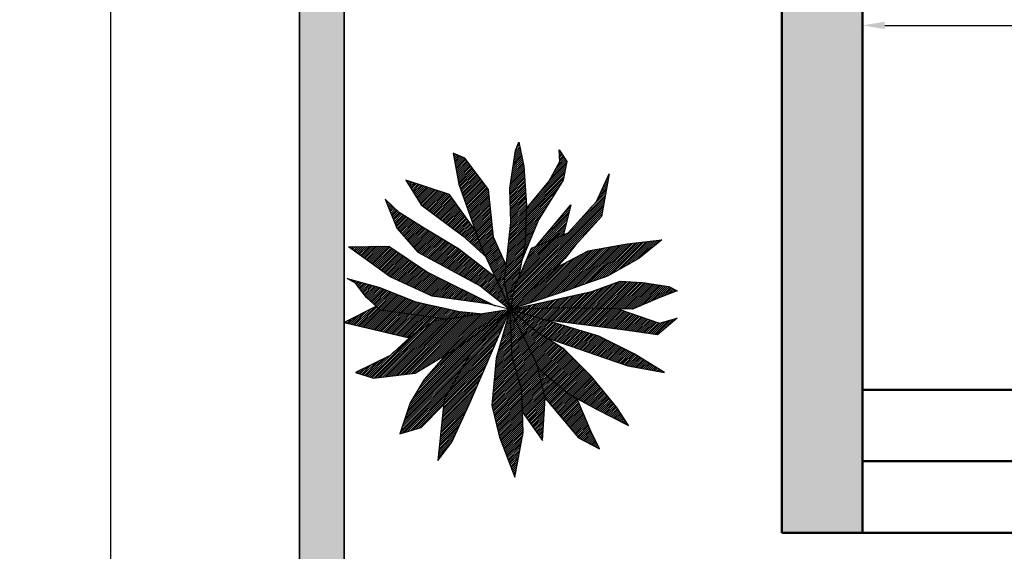
# Model space of a CAD drawing. Units: inches. Extents: x 3008 to 4088, y 1255 to 2137.
# Tile 3 of 30: x 3008 to 3119, y 1539 to 1598. Entities that reach past the tile are written whole.
import ezdxf

# ---------------------------------------------------------------- set-up
doc = ezdxf.new("R2010")
doc.units = ezdxf.units.IN
for name, color, linetype, lineweight in [('A-ANNO-DIMS', 2, 'Continuous', 18), ('A-WALL', 7, 'Continuous', 50), ('A-WALL-PATT', 8, 'Continuous', 13), ('C-PROP', 1, 'Continuous', 35), ('C-PROP-PATT', 9, 'Continuous', 13), ('L-PLNT', 3, 'Continuous', 13), ('vfolhas', 114, 'Continuous', 5)]:
    doc.layers.add(name, color=color, linetype=linetype, lineweight=lineweight)
for name, color, linetype in [('vfolha', 72, 'Continuous'), ('vfolha2', 110, 'Continuous'), ('vfolhas2', 102, 'Continuous')]:
    doc.layers.add(name, color=color, linetype=linetype)
doc.styles.get("Standard").update_dxf_attribs({"font": 'arial.ttf'})
doc.dimstyles.new('ISO-25', dxfattribs={"dimtxt": 8, "dimasz": 2.5, "dimexe": 1.25, "dimexo": 0.625, "dimtad": 1, "dimdec": 1, "dimlunit": 3, "dimtxsty": 'Standard', "dimcen": 2.5, "dimadec": 0, "dimazin": 0, "dimtfac": 1, "dimtdec": 1, "dimtmove": 0, "dimatfit": 3, "dimfxl": 1, "dimarcsym": 0})
pattern_1 = [(45, (-2446.5133113, 50.986076), (-0.004419417382, 0.004419417382), [])]

# ---------------------------------------------------------------- blocks, each defined once
blk = doc.blocks.new('*D2')
at = {"layer": 'A-ANNO-DIMS', "color": 0, "lineweight": -2, "transparency": 16777216}
for p, q in [((3039.04, 2003.97), (3017.26, 2003.97)), ((3018.51, 2001.47), (3018.51, 1346.47)), ((3039.04, 1343.97), (3017.26, 1343.97))]:
    blk.add_line(p, q, dxfattribs=at)
at = {"layer": 'A-ANNO-DIMS', "color": 0, "transparency": 16777216}
for points in [[(3018.09, 2001.47), (3018.93, 2001.47), (3018.51, 2003.97)], [(3018.09, 1346.47), (3018.93, 1346.47), (3018.51, 1343.97)]]:
    blk.add_solid(points, dxfattribs=at)
at = {"layer": 'Defpoints', "color": 0, "transparency": 16777216}
for p in [(3039.67, 2003.97), (3018.51, 1343.97), (3039.67, 1343.97)]:
    blk.add_point(p, dxfattribs=at)
at = {"layer": 'A-ANNO-DIMS', "color": 0, "transparency": 16777216, "insert": (3013.82, 1673.97), "char_height": 8, "attachment_point": 5, "rotation": 90}
blk.add_mtext("55'", dxfattribs=at)
blk = doc.blocks.new('arbusto_PB_verde_grande')
at = {"layer": 'vfolha2'}
h = blk.add_hatch(dxfattribs=at)
h.set_pattern_fill('ANSI31', color=256, scale=0.05, style=0)
h.set_pattern_definition(pattern_1)
h.paths.add_polyline_path([(0.0294, 0.3565), (0.0003, 0.0905), (0.0263, -0.0393), (0.047, 0.0623), (0.0619, 0.0973), (0.0937, 0.2657), (0.0996, 0.4347), (0.0879, 0.6131), (0.0645, 0.7227), (0.0499, 0.6851), (0.0236, 0.5129)])
h.paths.add_polyline_path([(0.3011, 0.4379), (0.1423, 0.2487), (0.2669, 0.3002)])
h.paths.add_polyline_path([(0.38, 0.2282), (0.237, 0.1519), (0.1843, 0.0936), (0.1112, 0.0436), (0.0263, -0.0393), (0.2806, 0.0467), (0.3683, 0.078), (0.4676, 0.1124), (0.6107, 0.1938), (0.7159, 0.2782), (0.5581, 0.2595)])
h.paths.add_polyline_path([(0.561, -0.2944), (0.7275, -0.3257), (0.5902, -0.2412), (0.4296, -0.1598), (0.0263, -0.0393), (0.1492, -0.1411), (0.1884, -0.166), (0.415, -0.2444)])
h.paths.add_polyline_path([(-0.2743, -0.4478), (-0.3035, -0.7263), (-0.2392, -0.6417), (-0.1546, -0.4572), (0.0263, -0.0393), (-0.1633, -0.2538)])
h.paths.add_polyline_path([(-0.5196, -0.2474), (-0.6774, -0.3257), (-0.5956, -0.3507), (-0.4057, -0.3288), (-0.2101, -0.21), (0.0263, -0.0393), (-0.1487, -0.0659), (-0.3152, -0.091), (-0.4145, -0.1505)])
h.paths.add_polyline_path([(-0.5255, 0.2501), (-0.7095, 0.247), (-0.5196, 0.1093), (-0.3298, 0.0217), (-0.0757, -0.0128), (-0.0423, -0.0215), (-0.3502, 0.1312)])
h = blk.add_hatch(dxfattribs=at)
h.set_pattern_fill('ANSI31', color=256, scale=0.05, style=0)
h.set_pattern_definition(pattern_1)
h.paths.add_polyline_path([(-0.1896, 0.297), (-0.0855, 0.2019), (-0.1078, 0.2501), (-0.132, 0.3187), (-0.251, 0.4848), (-0.4495, 0.5505), (-0.3795, 0.4379)])
h.paths.add_polyline_path([(0.0791, -0.4071), (0.0821, -0.5063), (0.1726, -0.6355), (0.1843, -0.4415), (0.149, -0.2918), (0.0263, -0.0393), (0.0353, -0.2538)])
at = {"layer": 'vfolhas'}
h = blk.add_hatch(dxfattribs=at)
h.set_pattern_fill('ANSI31', color=256, scale=0.05, style=0)
h.set_pattern_definition(pattern_1)
h.paths.add_polyline_path([(-0.0728, 0.5067), (-0.1808, 0.6506), (-0.2334, 0.6725), (-0.2071, 0.5318), (-0.1078, 0.2501), (0.0263, -0.0393), (0.0003, 0.0905), (0.0082, 0.1624), (-0.0494, 0.2908)])
h.paths.add_polyline_path([(0.099, 0.4193), (0.0937, 0.2657), (0.0791, 0.1881), (0.1551, 0.369), (0.2661, 0.5505), (0.2836, 0.635), (0.2485, 0.6882), (0.2514, 0.635), (0.2018, 0.5443)])
h.paths.add_polyline_path([(0.1229, 0.2407), (0.047, 0.0623), (0.0263, -0.0393), (0.1112, 0.0436), (0.1843, 0.0936), (0.2748, 0.1938), (0.3215, 0.2532), (0.4413, 0.3847), (0.4763, 0.5787), (0.4179, 0.4535), (0.2894, 0.3095)])
h.paths.add_polyline_path([(0.5815, -0.0378), (0.7071, 0.0154), (0.7859, 0.0467), (0.748, 0.0655), (0.6282, 0.0842), (0.526, 0.0905), (0.3974, 0.0436), (0.0263, -0.0393), (0.2573, -0.0315), (0.4383, -0.0347)])
h.paths.add_polyline_path([(0.5202, -0.0365), (0.4383, -0.0347), (0.2573, -0.0315), (0.0263, -0.0393), (0.1796, -0.0852), (0.5377, -0.1317), (0.6954, -0.1536), (0.7859, -0.0785), (0.7041, -0.1004)])
h.paths.add_polyline_path([(0.2719, -0.2193), (0.1492, -0.1411), (0.0263, -0.0393), (0.1579, -0.3101), (0.2952, -0.4258), (0.4179, -0.4916), (0.564, -0.5667), (0.5114, -0.4853), (0.3946, -0.3414)])
h.paths.add_polyline_path([(-0.0582, -0.4759), (-0.0231, -0.6198), (0.047, -0.8013), (0.0849, -0.5979), (0.0791, -0.4071), (0.0353, -0.2538), (0.0263, -0.0393), (-0.0377, -0.26)])
h.paths.add_polyline_path([(-0.2422, 0.1405), (-0.1107, 0.0686), (0.0263, -0.0393), (-0.0423, 0.1087), (-0.2101, 0.2376), (-0.3649, 0.3314), (-0.4787, 0.4034), (-0.543, 0.4629), (-0.4904, 0.3314), (-0.3941, 0.2219)])
h = blk.add_hatch(dxfattribs=at)
h.set_pattern_fill('ANSI31', color=256, scale=0.05, style=0)
h.set_pattern_definition(pattern_1)
h.paths.add_polyline_path([(-0.5722, 0.0623), (-0.7153, 0.103), (-0.6774, 0.0811), (-0.6277, 0.0154), (-0.5635, -0.041), (-0.2646, -0.0834), (-0.1487, -0.0659), (-0.1015, -0.0588), (-0.2042, -0.0472), (-0.4028, -0.0034)])
h.paths.add_polyline_path([(-0.5635, -0.041), (-0.5828, -0.024), (-0.7299, -0.0973), (-0.4334, -0.1679), (-0.4145, -0.1505), (-0.3152, -0.091), (-0.2646, -0.0834)])
h.paths.add_polyline_path([(-0.2769, -0.4727), (-0.2743, -0.4478), (-0.1633, -0.2538), (0.0263, -0.0393), (-0.2101, -0.21), (-0.2672, -0.2447), (-0.3649, -0.357), (-0.4291, -0.4634), (-0.4759, -0.6043), (-0.3795, -0.576)])
h = blk.add_hatch(dxfattribs=at)
h.set_pattern_fill('ANSI31', color=256, scale=0.05, style=0)
h.set_pattern_definition(pattern_1)
h.paths.add_polyline_path([(0.3361, -0.623), (0.4325, -0.6731), (0.3946, -0.5948), (0.3303, -0.4446), (0.2952, -0.4258), (0.1579, -0.3101), (0.149, -0.2918), (0.1843, -0.4415)])
at = {"layer": 'vfolha'}
for p, q in [((0.0263, -0.0393), (-0.1487, -0.0659)), ((0.0263, -0.0393), (-0.0377, -0.26)), ((0.0353, -0.2538), (0.0263, -0.0393)), ((0.5202, -0.0365), (0.7041, -0.1004)), ((0.5377, -0.1317), (0.1796, -0.0852)), ((0.7859, -0.0785), (0.6954, -0.1536)), ((0.7041, -0.1004), (0.7859, -0.0785)), ((0.6954, -0.1536), (0.5377, -0.1317)), ((0.3946, -0.3414), (0.2719, -0.2193)), ((-0.2672, -0.2447), (-0.3649, -0.357)), ((-0.0377, -0.26), (-0.0582, -0.4759)), ((0.0791, -0.4071), (0.0353, -0.2538)), ((0.1579, -0.3101), (0.2952, -0.4258)), ((0.5114, -0.4853), (0.3946, -0.3414)), ((0.0849, -0.5979), (0.0791, -0.4071)), ((0.2952, -0.4258), (0.4179, -0.4916)), ((0.4179, -0.4916), (0.564, -0.5667)), ((0.564, -0.5667), (0.5114, -0.4853)), ((-0.0231, -0.6198), (0.047, -0.8013)), ((0.047, -0.8013), (0.0849, -0.5979))]:
    blk.add_line(p, q, dxfattribs=at)
at = {"layer": 'vfolha2'}
for p, q in [((0.0499, 0.6851), (0.0645, 0.7227)), ((0.0645, 0.7227), (0.0879, 0.6131)), ((0.0236, 0.5129), (0.0499, 0.6851)), ((0.0879, 0.6131), (0.0996, 0.4347)), ((-0.4495, 0.5505), (-0.3795, 0.4379)), ((-0.251, 0.4848), (-0.4495, 0.5505)), ((0.0294, 0.3565), (0.0236, 0.5129)), ((-0.132, 0.3187), (-0.251, 0.4848)), ((-0.3795, 0.4379), (-0.1896, 0.297)), ((0.0996, 0.4347), (0.0937, 0.2657)), ((0.1434, 0.2501), (0.3011, 0.4379)), ((0.3011, 0.4379), (0.2661, 0.297)), ((0.0003, 0.0905), (0.0294, 0.3565)), ((-0.1896, 0.297), (-0.0822, 0.1989)), ((0.5581, 0.2595), (0.7159, 0.2782)), ((0.7159, 0.2782), (0.6107, 0.1938)), ((-0.7095, 0.247), (-0.5255, 0.2501)), ((-0.5196, 0.1093), (-0.7095, 0.247)), ((-0.5255, 0.2501), (-0.3502, 0.1312)), ((0.237, 0.1519), (0.38, 0.2282)), ((0.38, 0.2282), (0.5581, 0.2595)), ((0.6107, 0.1938), (0.4676, 0.1124)), ((-0.3298, 0.0217), (-0.5196, 0.1093)), ((-0.3502, 0.1312), (-0.0423, -0.0215)), ((0.0263, -0.0393), (0.0003, 0.0905)), ((0.2806, 0.0467), (0.0263, -0.0393)), ((0.3683, 0.078), (0.2806, 0.0467)), ((-0.0757, -0.0128), (-0.3298, 0.0217)), ((-0.2101, -0.21), (0.0263, -0.0393)), ((0.0263, -0.0393), (-0.1633, -0.2538)), ((-0.1546, -0.4572), (0.0263, -0.0393)), ((0.4296, -0.1598), (0.0263, -0.0393)), ((0.0263, -0.0393), (0.1579, -0.3101)), ((-0.1487, -0.0659), (-0.3152, -0.091)), ((-0.3152, -0.091), (-0.4145, -0.1505)), ((-0.4145, -0.1505), (-0.5196, -0.2474)), ((0.1884, -0.166), (0.415, -0.2444)), ((0.5902, -0.2412), (0.4296, -0.1598)), ((-0.4057, -0.3288), (-0.2101, -0.21)), ((-0.5196, -0.2474), (-0.6774, -0.3257)), ((-0.1633, -0.2538), (-0.2743, -0.4478)), ((0.415, -0.2444), (0.561, -0.2944)), ((0.7275, -0.3257), (0.5902, -0.2412)), ((0.1843, -0.4415), (0.149, -0.2918)), ((0.561, -0.2944), (0.7275, -0.3257)), ((-0.6774, -0.3257), (-0.5956, -0.3507)), ((-0.5956, -0.3507), (-0.4057, -0.3288)), ((-0.2743, -0.4478), (-0.3035, -0.7263)), ((0.1726, -0.6355), (0.1843, -0.4415)), ((0.0821, -0.5063), (0.1726, -0.6355)), ((-0.3035, -0.7263), (-0.2392, -0.6417))]:
    blk.add_line(p, q, dxfattribs=at)
at = {"layer": 'vfolhas2'}
for p, q in [((-0.2334, 0.6725), (-0.2071, 0.5318)), ((-0.1808, 0.6506), (-0.2334, 0.6725)), ((0.2514, 0.635), (0.2485, 0.6882)), ((0.2485, 0.6882), (0.2836, 0.635)), ((-0.0728, 0.5067), (-0.1808, 0.6506)), ((0.2018, 0.5443), (0.2514, 0.635)), ((0.2836, 0.635), (0.2661, 0.5505)), ((0.099, 0.4193), (0.2018, 0.5443)), ((0.2661, 0.5505), (0.1551, 0.369)), ((0.4179, 0.4535), (0.4763, 0.5787)), ((0.4763, 0.5787), (0.4413, 0.3847)), ((-0.2071, 0.5318), (-0.1078, 0.2501)), ((-0.0494, 0.2908), (-0.0728, 0.5067)), ((-0.543, 0.4629), (-0.4904, 0.3314)), ((-0.4787, 0.4034), (-0.543, 0.4629)), ((0.2894, 0.3095), (0.4179, 0.4535)), ((-0.3649, 0.3314), (-0.4787, 0.4034)), ((0.1551, 0.369), (0.078, 0.1855)), ((0.4413, 0.3847), (0.3215, 0.2532)), ((-0.4904, 0.3314), (-0.3941, 0.2219)), ((-0.2101, 0.2376), (-0.3649, 0.3314)), ((0.0082, 0.1624), (-0.0494, 0.2908)), ((0.1229, 0.2407), (0.2894, 0.3095)), ((-0.0423, 0.1087), (-0.2101, 0.2376)), ((-0.1078, 0.2501), (0.0263, -0.0393)), ((0.047, 0.0623), (0.1229, 0.2407)), ((0.0937, 0.2657), (0.0619, 0.0973)), ((0.3215, 0.2532), (0.2748, 0.1938)), ((-0.3941, 0.2219), (-0.2422, 0.1405)), ((0.2748, 0.1938), (0.1843, 0.0936)), ((-0.2422, 0.1405), (-0.1107, 0.0686)), ((-0.6774, 0.0811), (-0.7153, 0.103)), ((-0.7153, 0.103), (-0.5722, 0.0623)), ((0.1843, 0.0936), (0.1112, 0.0436)), ((0.4676, 0.1124), (0.3683, 0.078)), ((0.3974, 0.0436), (0.526, 0.0905)), ((0.526, 0.0905), (0.6282, 0.0842)), ((-0.6277, 0.0154), (-0.6774, 0.0811)), ((-0.5722, 0.0623), (-0.4028, -0.0034)), ((-0.1107, 0.0686), (0.0263, -0.0393)), ((0.0263, -0.0393), (0.047, 0.0623)), ((0.6282, 0.0842), (0.748, 0.0655)), ((0.7859, 0.0467), (0.7071, 0.0154)), ((0.748, 0.0655), (0.7859, 0.0467)), ((-0.5635, -0.041), (-0.6277, 0.0154)), ((0.0263, -0.0393), (0.3974, 0.0436)), ((0.1112, 0.0436), (0.0263, -0.0393)), ((0.7071, 0.0154), (0.5815, -0.0378)), ((-0.5828, -0.024), (-0.7299, -0.0973)), ((-0.2646, -0.0834), (-0.5635, -0.041)), ((-0.4028, -0.0034), (-0.2042, -0.0472)), ((0.0263, -0.0393), (-0.0757, -0.0128)), ((0.2573, -0.0315), (0.0263, -0.0393)), ((0.1492, -0.1411), (0.0263, -0.0393)), ((0.4383, -0.0347), (0.2573, -0.0315)), ((0.5815, -0.0378), (0.4383, -0.0347)), ((-0.2042, -0.0472), (-0.0983, -0.0591)), ((-0.7299, -0.0973), (-0.4334, -0.1679)), ((0.2719, -0.2193), (0.1492, -0.1411)), ((-0.3649, -0.357), (-0.4291, -0.4634)), ((0.1843, -0.4415), (0.3361, -0.623)), ((0.3946, -0.5948), (0.329, -0.4417)), ((-0.4291, -0.4634), (-0.4759, -0.6043)), ((-0.3795, -0.576), (-0.2769, -0.4727)), ((-0.2392, -0.6417), (-0.1546, -0.4572)), ((-0.0582, -0.4759), (-0.0231, -0.6198)), ((-0.4759, -0.6043), (-0.3795, -0.576)), ((0.3361, -0.623), (0.4325, -0.6731)), ((0.4325, -0.6731), (0.3946, -0.5948))]:
    blk.add_line(p, q, dxfattribs=at)
blk = doc.blocks.new('*D43')
at = {"layer": 'A-ANNO-DIMS', "color": 0, "lineweight": -2, "transparency": 16777216}
for p, q in [((3102.67, 1604.34), (3102.67, 1596.52)), ((3150.67, 1604.34), (3150.67, 1596.52)), ((3105.17, 1597.77), (3148.17, 1597.77)), ((3150.67, 1597.77), (3242.99, 1597.77))]:
    blk.add_line(p, q, dxfattribs=at)
at = {"layer": 'A-ANNO-DIMS', "color": 0, "transparency": 16777216}
for points in [[(3105.17, 1598.18), (3105.17, 1597.35), (3102.67, 1597.77)], [(3148.17, 1598.18), (3148.17, 1597.35), (3150.67, 1597.77)]]:
    blk.add_solid(points, dxfattribs=at)
at = {"layer": 'Defpoints', "color": 0, "transparency": 16777216}
for p in [(3102.67, 1604.97), (3150.67, 1604.97), (3150.67, 1597.77)]:
    blk.add_point(p, dxfattribs=at)
at = {"layer": 'A-ANNO-DIMS', "color": 0, "transparency": 16777216, "insert": (3198.08, 1602.53), "char_height": 8, "attachment_point": 5}
blk.add_mtext('MAIN DOOR 4\'-0"', dxfattribs=at)

msp = doc.modelspace()

# ---------------------------------------------------------------- hatches: boundary and pattern name
at = {"layer": 'A-WALL-PATT'}
h = msp.add_hatch(color=256, dxfattribs=at)
h.dxf.hatch_style = 1
h.paths.add_polyline_path([(3102.67, 1625.97), (3093.67, 1625.97), (3093.67, 1540.97), (3102.67, 1540.97)])
h.paths.add_polyline_path([(3102.67, 1784.97), (3252.67, 1784.97), (3252.67, 1790.97), (3102.67, 1790.97), (3102.67, 1892.97), (3093.67, 1892.97), (3093.67, 1667.97), (3102.67, 1667.97)])
h.paths.add_polyline_path([(3192.67, 1943.97), (3093.67, 1943.97), (3093.67, 1934.97), (3102.67, 1934.97), (3192.67, 1934.97)])
h.paths.add_polyline_path([(3264.67, 1943.97), (3234.67, 1943.97), (3234.67, 1934.97), (3246.67, 1934.97), (3246.67, 1868.97), (3252.67, 1868.97), (3252.67, 1934.97), (3264.67, 1934.97)])
h.paths.add_polyline_path([(3330.67, 1943.97), (3288.67, 1943.97), (3288.67, 1934.97), (3300.67, 1934.97), (3300.67, 1838.97), (3246.67, 1838.97), (3246.67, 1826.97), (3252.67, 1826.97), (3252.67, 1832.97), (3306.67, 1832.97), (3306.67, 1934.97), (3330.67, 1934.97)])
h.paths.add_polyline_path([(3390.67, 1943.97), (3360.67, 1943.97), (3360.67, 1934.97), (3390.67, 1934.97)])
h.paths.add_polyline_path([(3465.67, 1943.97), (3432.67, 1943.97), (3432.67, 1934.97), (3456.67, 1934.97), (3456.67, 1883.97), (3465.67, 1883.97)])
h.paths.add_polyline_path([(3465.67, 1841.97), (3456.67, 1841.97), (3456.67, 1790.97), (3370.67, 1790.97), (3370.67, 1784.97), (3456.67, 1784.97), (3456.67, 1759.47), (3465.67, 1759.47)])
h.paths.add_polyline_path([(3465.67, 1693.47), (3456.67, 1693.47), (3456.67, 1667.97), (3330.67, 1667.97), (3330.67, 1643.97), (3336.67, 1643.97), (3336.67, 1661.97), (3456.67, 1661.97), (3456.67, 1649.97), (3465.67, 1649.97)])
h.paths.add_polyline_path([(3465.67, 1625.97), (3456.67, 1625.97), (3456.67, 1613.97), (3324.67, 1613.97), (3324.67, 1604.97), (3456.67, 1604.97), (3456.67, 1571.97), (3465.67, 1571.97)])
h.paths.add_polyline_path([(3465.67, 1505.97), (3456.67, 1505.97), (3456.67, 1472.97), (3438.67, 1472.97), (3438.67, 1463.97), (3465.67, 1463.97)])
h.paths.add_polyline_path([(3396.67, 1472.97), (3354.67, 1472.97), (3354.67, 1463.97), (3396.67, 1463.97)])
h.paths.add_polyline_path([(3312.67, 1472.97), (3288.67, 1472.97), (3288.67, 1550.97), (3282.67, 1550.97), (3282.67, 1472.97), (3270.67, 1472.97), (3270.67, 1463.97), (3312.67, 1463.97)])
h.paths.add_polyline_path([(3246.67, 1472.97), (3234.67, 1472.97), (3234.67, 1544.97), (3252.67, 1544.97), (3252.67, 1550.97), (3234.67, 1550.97), (3234.67, 1604.97), (3282.67, 1604.97), (3282.67, 1580.97), (3288.67, 1580.97), (3288.67, 1613.97), (3150.67, 1613.97), (3150.67, 1604.97), (3225.67, 1604.97), (3225.67, 1463.97), (3246.67, 1463.97)])
at = {"layer": 'C-PROP-PATT'}
h = msp.add_hatch(color=256, dxfattribs=at)
h.dxf.hatch_style = 1
h.paths.add_polyline_path([(3519.67, 2003.97), (3039.67, 2003.97), (3039.67, 1343.97), (3051.67, 1343.97), (3051.67, 1348.97), (3044.67, 1348.97), (3044.67, 1998.97), (3514.67, 1998.97), (3514.67, 1348.97), (3219.67, 1348.97), (3219.67, 1343.97), (3519.67, 1343.97)])

# ---------------------------------------------------------------- linework, layer by layer
at = {"layer": 'A-WALL'}
for p, q in [((3093.67, 1540.97), (3093.67, 1943.97)), ((3102.67, 1540.97), (3102.67, 1784.97)), ((3102.67, 1556.97), (3225.67, 1556.97)), ((3102.67, 1548.97), (3225.67, 1548.97)), ((3225.67, 1540.97), (3093.67, 1540.97))]:
    msp.add_line(p, q, dxfattribs=at)
at = {"layer": 'C-PROP'}
for p, q in [((3039.67, 1343.97), (3039.67, 2003.97)), ((3044.67, 1348.97), (3044.67, 1998.97))]:
    msp.add_line(p, q, dxfattribs=at)

# ---------------------------------------------------------------- block references
at = {"layer": 'L-PLNT', "xscale": 24.60366729364114, "yscale": 24.60366729364114, "zscale": 24.60366729364114}
msp.add_blockref('arbusto_PB_verde_grande', (3062.62, 1566.91), dxfattribs=at)

# ---------------------------------------------------------------- dimensions: what is measured, and where the dimension line sits
at = {"layer": 'A-ANNO-DIMS'}
dim = msp.add_linear_dim(base=(3018.51, 1343.97), p1=(3039.67, 2003.97), p2=(3039.67, 1343.97), angle=90, dimstyle='ISO-25', override={"dimclrd": 0, "dimclre": 0, "dimclrt": 0}, dxfattribs=at)
dim.commit()
dim.dimension.update_dxf_attribs({"geometry": '*D2', "text_midpoint": (3013.82, 1673.97)})
dim = msp.add_linear_dim(base=(3150.67, 1597.77), p1=(3102.67, 1604.97), p2=(3150.67, 1604.97), text='MAIN DOOR <>', dimstyle='ISO-25', override={"dimdec": 1, "dimrnd": 0, "dimzin": 1, "dimlunit": 4, "dimfrac": 2}, dxfattribs=at)
dim.commit()
dim.dimension.update_dxf_attribs({"geometry": '*D43', "text_midpoint": (3198.08, 1602.53)})

doc.saveas('drawing.dxf')
